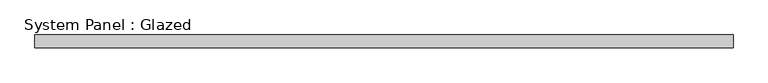
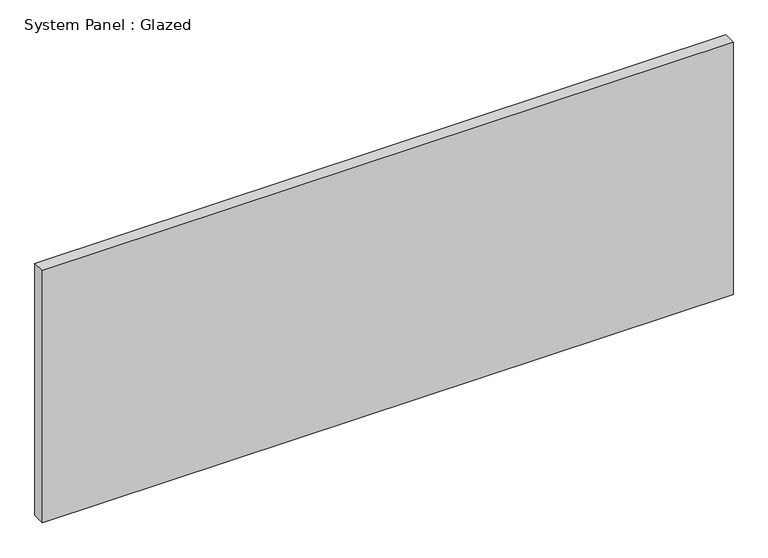
"""IFC4 building model written with IfcOpenShell, lengths in millimetres: plate geometry, System Panel : Glazed."""

from ifc_helpers import new_model, si_unit, origin, origin_with_axes, place, context, project, spatial, polyline, outline, extrude, source, transform, mapped, element, save


def system_panel_glazed_43256be5(model_context):
    return source(origin(), model_context, "Body", "SweptSolid", [
        extrude(outline(polyline([(688.975, 19.05), (-688.975, 19.05), (-688.975, 44.45), (688.975, 44.45), (688.975, 19.05)])), origin_with_axes(), (0.0, 0.0, 1.0), 532.0236621),
    ])


if __name__ == "__main__":
    model = new_model("IFC4")
    model_context = context("Model", 3, world=origin())
    ifc_project = project(units=[si_unit("LENGTHUNIT", "METRE", prefix="MILLI")], contexts=[model_context])
    site = spatial("IfcSite", under=ifc_project)
    building = spatial("IfcBuilding", under=site)
    placement = place(None, origin())
    system_panel_glazed_shape = system_panel_glazed_43256be5(model_context)
    element("IfcPlate", 1, ObjectType="System Panel : Glazed", at=placement, inside=building, context=model_context, shape_type="MappedRepresentation", body=[
        mapped(system_panel_glazed_shape, transform((0.0, 0.0, 0.0), x_axis=(1.0, 0.0, 0.0), y_axis=(0.0, 1.0, 0.0), z_axis=(0.0, 0.0, 1.0))),
    ])
    save(model, "model.ifc")

# Revit data of these elements
# Type "System Panel : Glazed"
#   Construction Type Id = "GSP4R"
#   Analytic Construction = "1/8 in Pilkington single glazing"
#   Visual Light Transmittance = 0.9
#   Solar Heat Gain Coefficient = 0.86
#   Heat Transfer Coefficient (U) = 1.18115 BTU/(h·ft²·°F)
#   Define Thermal Properties by = 1
# Element 1 (IfcPlate, "System Panel : Glazed")
#   Materials on its faces: "Glass"
# Materials
#   "Glass": class "Glass", colour RGB 0 128 192, transparency 0.75, Description = "Soda Lime Glass", Cost = 0
